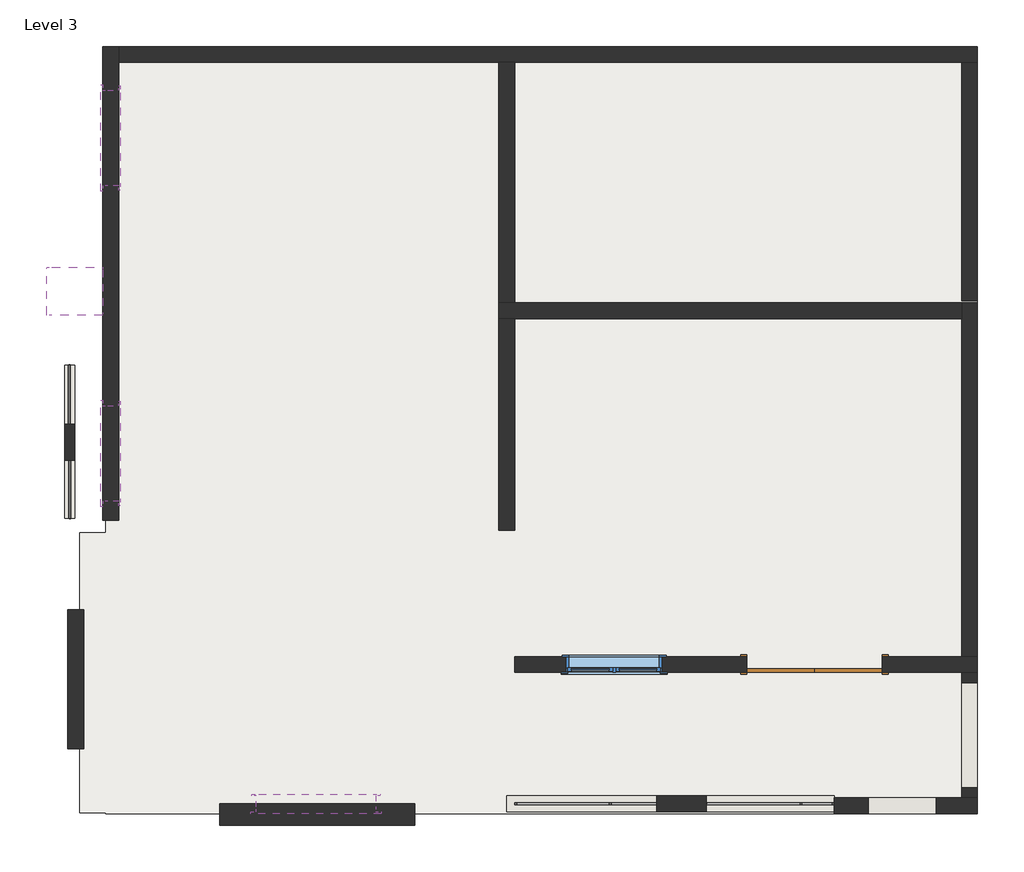
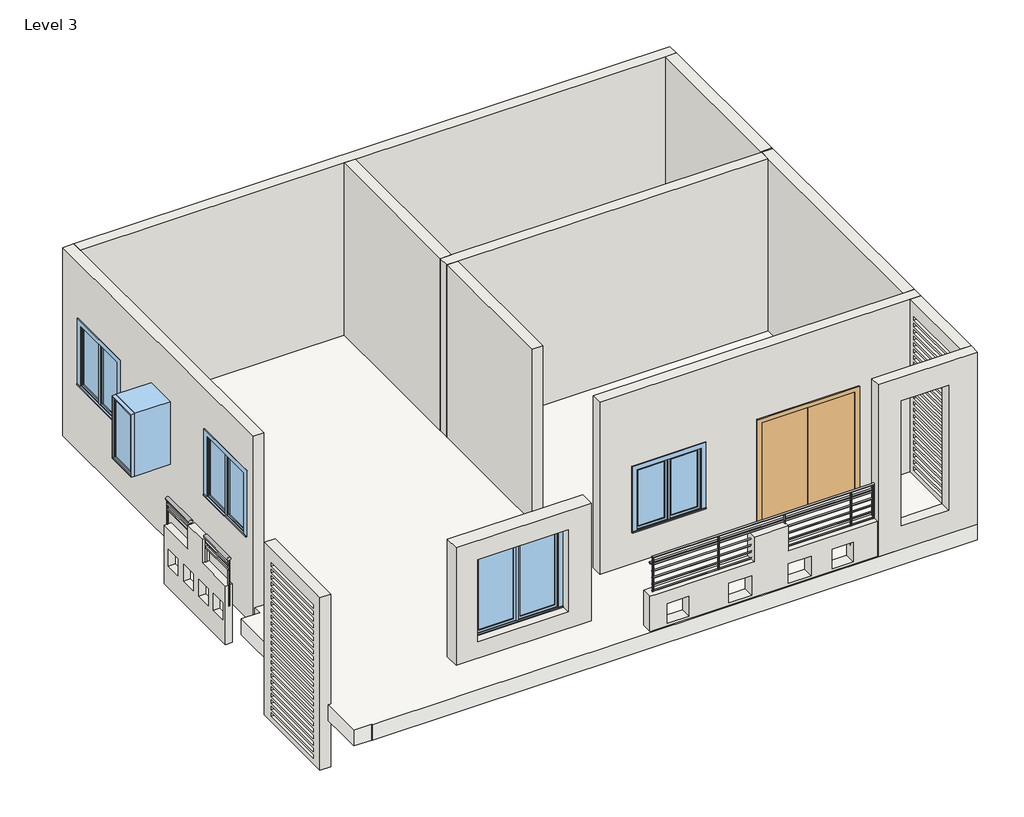
# One storey: 14 walls, 5 windows, 3 railings, 1 door, 1 roof.
# Revit data of these elements (continued)
# Element 16 (IfcWall, "Generic - 8\"") (continued)
#   Base Constraint = Level 3
#   Materials on its faces: "Default Wall"
# Element 17 (IfcWall, "Generic - 8\"")
#   built-in parameter 1001111 = 1' - 0"
#   Top Offset = 0' - 0"
#   Base Offset = 1' - 0"
#   Unconnected Height = 4' - 0"
#   wall height = 4' - 0"
#   Phase Created = New Construction
#   Base Constraint = Level 3
#   Materials on its faces: "Default Wall"
# Element 18 (IfcWall, "Generic - 8\"")
#   built-in parameter 1001111 = -3' - 0"
#   Top Offset = 0' - 0"
#   Base Offset = -3' - 0"
#   Unconnected Height = 11' - 0.09429"
#   wall height = 11' - 0.09429"
#   Phase Created = New Construction
#   Base Constraint = Level 3
#   Materials on its faces: "Default Wall"
# Element 19 (IfcWall, "Walls 3 : Walls 1")
#   Phase Created = New Construction
#   Materials on its faces: "Default Wall"
# Element 20 (IfcWindow, "Casement Dbl with Trim : 48\" x 48\"")
#   Mark = "4"
#   Phase Created = New Construction
#   Materials on its faces: "Sash", "Trim", "Glass"
# Element 21 (IfcWindow, "Casement Dbl with Trim : 48\" x 48\"")
#   Mark = "6"
#   Phase Created = New Construction
#   Materials on its faces: "Sash", "Trim", "Glass"
# Element 22 (IfcWindow, "Casement Dbl with Trim : 48\" x 48\"")
#   Mark = "10"
#   Phase Created = New Construction
#   Materials on its faces: "Sash", "Trim", "Glass"
# Element 23 (IfcWindow, "Casement Dbl with Trim.0001 : 60\" x 60\"")
#   Mark = "2"
#   Phase Created = New Construction
#   Materials on its faces: "Sash", "Trim", "Glass"
# Element 24 (IfcWindow, "Fixed : 24\" x 48\"")
#   Mark = "8"
#   Phase Created = New Construction
#   Materials on its faces: "Sash", "Glass"
# Materials
#   "Wood - Birch - Solid Stained Light Low Gloss": class "Wood", colour RGB 210 159 95, transparency 0, Cost = 0
#   "Paint - Sienna": colour RGB 118 70 51, transparency 0, Cost = 0
#   "Glass": class "Glass", colour RGB 0 128 192, transparency 0.75, Description = "Soda Lime Glass", Cost = 0
#   "Sash": class "Wood", colour RGB 224 178 126, transparency 0
#   "Trim": class "Wood", colour RGB 224 178 126, transparency 0
#   "Default Roof": colour RGB 88 101 114, transparency 0
#   "Default Wall": colour RGB 128 128 128, transparency 0
